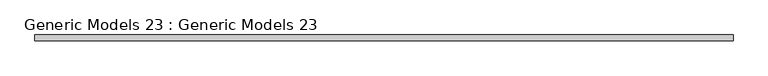
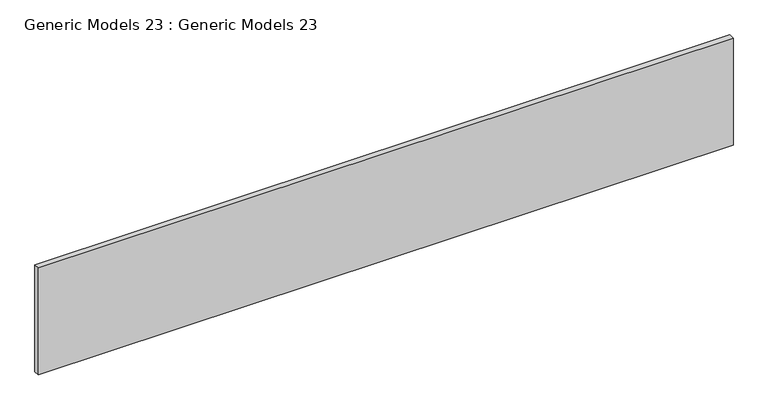
"""IFC4 building model written with IfcOpenShell, lengths in millimetres: proxy geometry, Generic Models 23 : Generic Models 23."""

from ifc_helpers import new_model, si_unit, frame, origin, place, context, project, spatial, polyline, outline, extrude, source, transform, mapped, element, save


def generic_models_23_generic_models_23_7b700280(model_context):
    return source(origin(), model_context, "Body", "SweptSolid", [
        extrude(outline(polyline([(-5026.5586008, -7500.7844117), (-11107.9539306, -7500.7844117), (-11107.9539306, -7449.9844117), (-5026.5586008, -7449.9844117), (-5026.5586008, -7500.7844117)])), frame((0.0, 0.0, 3124.2), z_axis=(0.0, 0.0, 1.0), x_axis=(1.0, 0.0, 0.0)), (0.0, 0.0, 1.0), 990.6),
    ])


if __name__ == "__main__":
    model = new_model("IFC4")
    model_context = context("Model", 3, world=origin())
    ifc_project = project(units=[si_unit("LENGTHUNIT", "METRE", prefix="MILLI")], contexts=[model_context])
    site = spatial("IfcSite", under=ifc_project)
    building = spatial("IfcBuilding", under=site)
    placement = place(None, origin())
    generic_models_23_generic_models_23_shape = generic_models_23_generic_models_23_7b700280(model_context)
    element("IfcBuildingElementProxy", 1, Name="Generic Models 23 : Generic Models 23", ObjectType="Generic Models 23 : Generic Models 23", at=placement, inside=building, context=model_context, shape_type="MappedRepresentation", body=[
        mapped(generic_models_23_generic_models_23_shape, transform((0.0, 0.0, 0.0), x_axis=(1.0, 0.0, 0.0), y_axis=(0.0, 1.0, 0.0), z_axis=(0.0, 0.0, 1.0))),
    ])
    save(model, "model.ifc")

# Revit data of these elements
# Element 1 (IfcBuildingElementProxy, "Generic Models 23 : Generic Models 23")
#   Materials on its faces: "SAND STONE BEIGE CLADDING"
# Materials
#   "SAND STONE BEIGE CLADDING": class "Generic", colour RGB 120 120 120, transparency 0, Cost = 0
